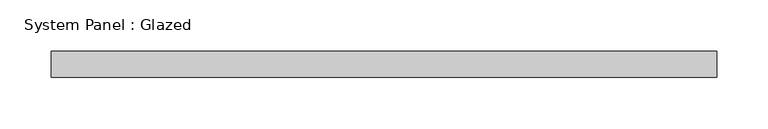
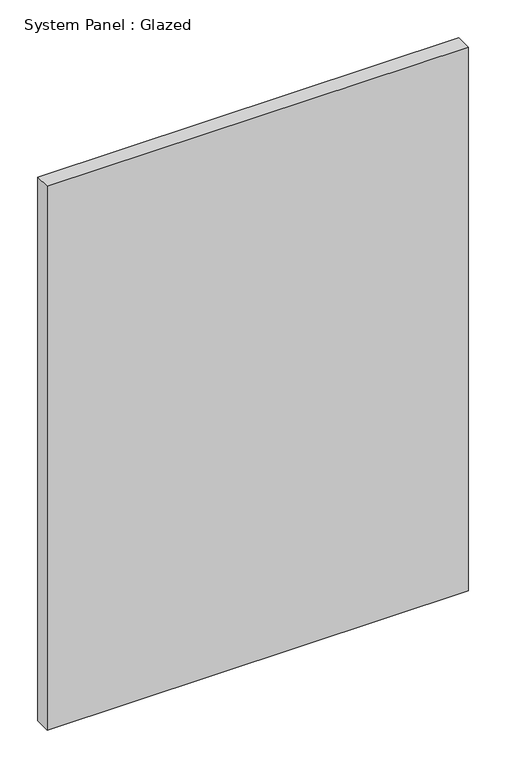
"""IFC4 building model written with IfcOpenShell, lengths in millimetres: plate geometry, System Panel : Glazed."""

from ifc_helpers import new_model, si_unit, origin, origin_with_axes, place, context, project, spatial, polyline, outline, extrude, source, transform, mapped, element, save


def system_panel_glazed_b409b60d(model_context):
    return source(origin(), model_context, "Body", "SweptSolid", [
        extrude(outline(polyline([(323.85, 19.05), (-323.85, 19.05), (-323.85, 44.45), (323.85, 44.45), (323.85, 19.05)])), origin_with_axes(), (0.0, 0.0, 1.0), 884.4809713),
    ])


if __name__ == "__main__":
    model = new_model("IFC4")
    model_context = context("Model", 3, world=origin())
    ifc_project = project(units=[si_unit("LENGTHUNIT", "METRE", prefix="MILLI")], contexts=[model_context])
    site = spatial("IfcSite", under=ifc_project)
    building = spatial("IfcBuilding", under=site)
    placement = place(None, origin())
    system_panel_glazed_shape = system_panel_glazed_b409b60d(model_context)
    element("IfcPlate", 1, ObjectType="System Panel : Glazed", at=placement, inside=building, context=model_context, shape_type="MappedRepresentation", body=[
        mapped(system_panel_glazed_shape, transform((0.0, 0.0, 0.0), x_axis=(1.0, 0.0, 0.0), y_axis=(0.0, 1.0, 0.0), z_axis=(0.0, 0.0, 1.0))),
    ])
    save(model, "model.ifc")

# Revit data of these elements
# Type "System Panel : Glazed"
#   Construction Type Id = "GSP4R"
#   Analytic Construction = "1/8 in Pilkington single glazing"
#   Visual Light Transmittance = 0.9
#   Solar Heat Gain Coefficient = 0.86
#   Heat Transfer Coefficient (U) = 1.18115 BTU/(h·ft²·°F)
#   Define Thermal Properties by = 1
# Element 1 (IfcPlate, "System Panel : Glazed")
#   Materials on its faces: "Glass"
# Materials
#   "Glass": class "Glass", colour RGB 0 128 192, transparency 0.75, Description = "Soda Lime Glass", Cost = 0
